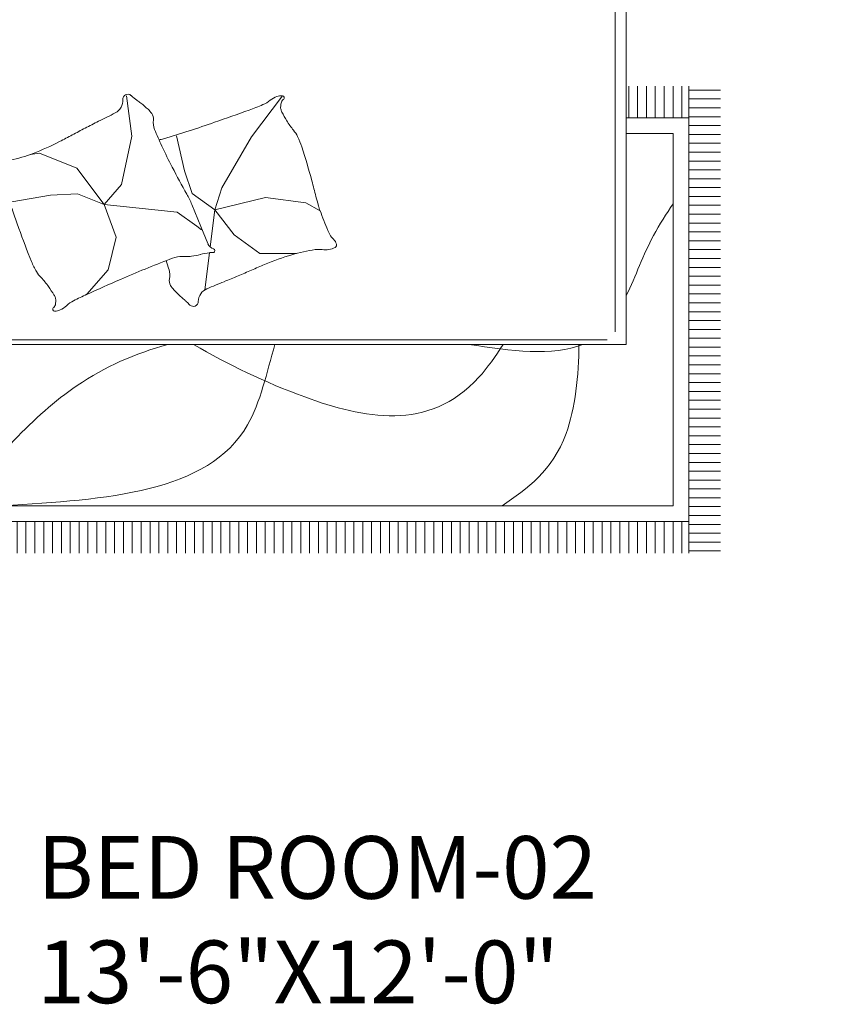
# Model space of a CAD drawing. Units: inches. Extents: x -7 to 1228, y -146 to 1091.
# Tile 30 of 88: x 680 to 744, y 367 to 446. Entities that reach past the tile are written whole.
import ezdxf

# ---------------------------------------------------------------- set-up
doc = ezdxf.new("R2010")
doc.units = ezdxf.units.IN
doc.layers.add('A-AREA-IDEN', color=7, linetype='Continuous', lineweight=18)
doc.layers.add('A-FURN', color=8, linetype='Continuous', lineweight=18)
doc.styles.add('DIM_FONT', font='SIMPLEX.shx', dxfattribs={"width": 0.8})
doc.styles.get("Standard").update_dxf_attribs({"font": 'arial.ttf'})

# ---------------------------------------------------------------- blocks, each defined once
blk = doc.blocks.new('A$C4F634EDD')
for p, q in [((0, 2.6295), (0, 2.2295)), ((0.5, 2.6295), (0, 2.6295)), ((0.5, 2.6295), (2.3, 2.6295)), ((0.5, 0.5295), (0.5, 2.6295)), ((0.5, 2.2295), (0.5, 2.6295)), ((2.3, 2.6295), (2.3, 0.5295)), ((2.3, 2.6295), (2.8, 2.6295)), ((2.3, 2.2295), (2.3, 2.6295)), ((2.8, 2.6295), (2.8, 2.2295)), ((0.5, 2.5771), (2.3, 2.5771)), ((2.392, 2.5115), (2.5692, 2.5765)), ((2.5692, 2.5765), (2.574, 2.5743)), ((0.2457, 2.5697), (0.2457, 2.4733)), ((2.4985, 2.5445), (2.5516, 2.564)), ((2.5062, 2.5454), (2.5487, 2.561)), ((2.5483, 2.5347), (2.5487, 2.561)), ((2.5487, 2.561), (2.5571, 2.56)), ((2.5615, 2.5536), (2.5514, 2.5318)), ((2.5516, 2.564), (2.5637, 2.5584)), ((2.5571, 2.56), (2.5615, 2.5536)), ((2.5615, 2.5536), (2.5791, 2.5058)), ((2.5637, 2.5584), (2.6418, 2.3458)), ((2.574, 2.5743), (2.6638, 2.3298)), ((2.4946, 2.5331), (2.4985, 2.5445)), ((2.5734, 2.3187), (2.4946, 2.5331)), ((2.5062, 2.5454), (2.5004, 2.5392)), ((2.5004, 2.5392), (2.5013, 2.5315)), ((2.5013, 2.5315), (2.5188, 2.4836)), ((2.5013, 2.5315), (2.5231, 2.5214)), ((2.5235, 2.5256), (2.5062, 2.5454)), ((2.5231, 2.5214), (2.5235, 2.5256)), ((2.5483, 2.5347), (2.5235, 2.5256)), ((2.5514, 2.5318), (2.5483, 2.5347)), ((2.5807, 2.4521), (2.5514, 2.5318)), ((2.3898, 2.5066), (2.392, 2.5115)), ((2.4795, 2.2621), (2.3898, 2.5066)), ((2.412, 2.5007), (2.4634, 2.5196)), ((2.4361, 2.4352), (2.412, 2.5007)), ((2.4634, 2.5196), (2.4875, 2.454)), ((2.4842, 2.5232), (2.47, 2.518)), ((2.47, 2.518), (2.472, 2.5127)), ((2.472, 2.5127), (2.4862, 2.5179)), ((2.4881, 2.5126), (2.4739, 2.5074)), ((2.4739, 2.5074), (2.4759, 2.502)), ((2.4759, 2.502), (2.4901, 2.5073)), ((2.492, 2.5019), (2.4778, 2.4967)), ((2.4862, 2.5179), (2.4842, 2.5232)), ((2.4901, 2.5073), (2.4881, 2.5126)), ((2.494, 2.4966), (2.492, 2.5019)), ((2.5523, 2.4417), (2.5231, 2.5214)), ((2.5791, 2.5058), (2.5788, 2.4956)), ((2.4778, 2.4967), (2.4798, 2.4914)), ((2.4798, 2.4914), (2.494, 2.4966)), ((2.4959, 2.4913), (2.4817, 2.4861)), ((2.4817, 2.4861), (2.4837, 2.4808)), ((2.4837, 2.4808), (2.4979, 2.486)), ((2.4998, 2.4807), (2.4856, 2.4755)), ((2.4856, 2.4755), (2.4876, 2.4702)), ((2.4876, 2.4702), (2.5018, 2.4754)), ((2.4979, 2.486), (2.4959, 2.4913)), ((2.5018, 2.4754), (2.4998, 2.4807)), ((2.5188, 2.4836), (2.5256, 2.4761)), ((2.5256, 2.4761), (2.5342, 2.4692)), ((2.5788, 2.4956), (2.5767, 2.4848)), ((2.5767, 2.4848), (2.5795, 2.4717)), ((2.4875, 2.454), (2.4361, 2.4352)), ((2.5037, 2.47), (2.4895, 2.4648)), ((2.4895, 2.4648), (2.4915, 2.4595)), ((2.4915, 2.4595), (2.5057, 2.4647)), ((2.5057, 2.4647), (2.5037, 2.47)), ((2.5342, 2.4692), (2.5405, 2.4574)), ((2.5405, 2.4574), (2.547, 2.4397)), ((2.5795, 2.4717), (2.586, 2.454)), ((2.5807, 2.4521), (2.6158, 2.3564)), ((2.5984, 2.4204), (2.586, 2.454)), ((2.4634, 2.4211), (2.474, 2.425)), ((2.474, 2.425), (2.4779, 2.4143)), ((2.4811, 2.4276), (2.4917, 2.4315)), ((2.485, 2.4169), (2.4811, 2.4276)), ((2.4917, 2.4315), (2.4956, 2.4208)), ((2.5594, 2.4061), (2.547, 2.4397)), ((2.5523, 2.4417), (2.5875, 2.346)), ((0.0957, 2.4197), (0.192, 2.4197)), ((0.2994, 2.4197), (0.3957, 2.4197)), ((2.4457, 2.4146), (2.4563, 2.4185)), ((2.4496, 2.4039), (2.4457, 2.4146)), ((2.4602, 2.4078), (2.4496, 2.4039)), ((2.4563, 2.4185), (2.4602, 2.4078)), ((2.4673, 2.4104), (2.4634, 2.4211)), ((2.4779, 2.4143), (2.4673, 2.4104)), ((2.4706, 2.4016), (2.4812, 2.4055)), ((2.4745, 2.3909), (2.4706, 2.4016)), ((2.4812, 2.4055), (2.4851, 2.3949)), ((2.4956, 2.4208), (2.485, 2.4169)), ((2.4883, 2.4081), (2.4989, 2.412)), ((2.4922, 2.3975), (2.4883, 2.4081)), ((2.5028, 2.4014), (2.4922, 2.3975)), ((2.4989, 2.412), (2.5028, 2.4014)), ((2.5622, 2.393), (2.5594, 2.4061)), ((2.6047, 2.4086), (2.5984, 2.4204)), ((2.6133, 2.4017), (2.6047, 2.4086)), ((2.6201, 2.3941), (2.6133, 2.4017)), ((2.4528, 2.3951), (2.4635, 2.399)), ((2.4567, 2.3844), (2.4528, 2.3951)), ((2.4674, 2.3883), (2.4567, 2.3844)), ((2.46, 2.3756), (2.4706, 2.3795)), ((2.4639, 2.365), (2.46, 2.3756)), ((2.4635, 2.399), (2.4674, 2.3883)), ((2.4706, 2.3795), (2.4745, 2.3689)), ((2.4851, 2.3949), (2.4745, 2.3909)), ((2.4777, 2.3821), (2.4883, 2.386)), ((2.4816, 2.3715), (2.4777, 2.3821)), ((2.4922, 2.3754), (2.4816, 2.3715)), ((2.4883, 2.386), (2.4922, 2.3754)), ((2.4954, 2.3886), (2.5061, 2.3925)), ((2.4993, 2.378), (2.4954, 2.3886)), ((2.51, 2.3819), (2.4993, 2.378)), ((2.5061, 2.3925), (2.51, 2.3819)), ((2.5238, 2.3769), (2.538, 2.3821)), ((2.5277, 2.3663), (2.5238, 2.3769)), ((2.538, 2.3821), (2.5419, 2.3715)), ((2.5598, 2.372), (2.5601, 2.3822)), ((2.5601, 2.3822), (2.5622, 2.393)), ((2.6376, 2.3463), (2.6201, 2.3941)), ((2.6499, 2.3979), (2.6397, 2.3953)), ((2.6417, 2.39), (2.6488, 2.391)), ((2.6488, 2.391), (2.6538, 2.3895)), ((2.6551, 2.397), (2.6499, 2.3979)), ((2.6538, 2.3895), (2.6596, 2.388)), ((2.6627, 2.392), (2.6551, 2.397)), ((2.6596, 2.388), (2.6626, 2.3867)), ((2.6626, 2.3867), (2.6662, 2.388)), ((2.6692, 2.394), (2.6627, 2.392)), ((2.6662, 2.388), (2.6632, 2.3828)), ((2.6632, 2.3828), (2.6736, 2.3744)), ((2.6736, 2.3944), (2.6692, 2.394)), ((2.6765, 2.391), (2.6736, 2.3944)), ((2.6742, 2.3795), (2.6765, 2.391)), ((2.6824, 2.3858), (2.6742, 2.3795)), ((2.6873, 2.3815), (2.6824, 2.3858)), ((2.6853, 2.369), (2.6873, 2.3815)), ((2.6946, 2.376), (2.6853, 2.369)), ((2.6995, 2.3713), (2.6946, 2.376)), ((0.2457, 2.366), (0.2457, 2.2697)), ((2.4745, 2.3689), (2.4639, 2.365)), ((2.4672, 2.3561), (2.4778, 2.36)), ((2.4711, 2.3455), (2.4672, 2.3561)), ((2.4778, 2.36), (2.4817, 2.3494)), ((2.4849, 2.3626), (2.4955, 2.3665)), ((2.4888, 2.352), (2.4849, 2.3626)), ((2.4994, 2.3559), (2.4888, 2.352)), ((2.4955, 2.3665), (2.4994, 2.3559)), ((2.5026, 2.3691), (2.5132, 2.373)), ((2.5065, 2.3585), (2.5026, 2.3691)), ((2.5171, 2.3624), (2.5065, 2.3585)), ((2.5132, 2.373), (2.5171, 2.3624)), ((2.5419, 2.3715), (2.5277, 2.3663)), ((2.5774, 2.3242), (2.5598, 2.372)), ((2.6154, 2.3522), (2.5905, 2.3431)), ((2.6158, 2.3564), (2.6154, 2.3522)), ((2.6154, 2.3522), (2.6327, 2.3324)), ((2.6376, 2.3463), (2.6158, 2.3564)), ((2.6736, 2.3744), (2.6922, 2.3593)), ((2.6922, 2.3593), (2.7051, 2.3473)), ((2.695, 2.3603), (2.6995, 2.3713)), ((2.7031, 2.3682), (2.695, 2.3603)), ((2.7096, 2.3616), (2.7031, 2.3682)), ((2.7062, 2.351), (2.7096, 2.3616)), ((2.7147, 2.3578), (2.7062, 2.351)), ((2.7214, 2.3517), (2.7147, 2.3578)), ((2.7196, 2.34), (2.7214, 2.3517)), ((0, 2.3301), (0.5, 2.3301)), ((2.8, 2.3301), (2.3, 2.3301)), ((2.4817, 2.3494), (2.4711, 2.3455)), ((2.5774, 2.3242), (2.5875, 2.346)), ((2.5875, 2.346), (2.5905, 2.3431)), ((2.5905, 2.3431), (2.5901, 2.3168)), ((2.613, 2.3312), (2.6077, 2.3293)), ((2.6077, 2.3293), (2.6135, 2.3141)), ((2.6192, 2.3174), (2.613, 2.3312)), ((2.6153, 2.3261), (2.6327, 2.3324)), ((2.6369, 2.332), (2.6161, 2.3243)), ((2.6616, 2.3249), (2.6234, 2.3109)), ((2.6327, 2.3324), (2.6385, 2.3386)), ((2.6418, 2.3458), (2.6369, 2.332)), ((2.6385, 2.3386), (2.6376, 2.3463)), ((2.6638, 2.3298), (2.6616, 2.3249)), ((2.7051, 2.3473), (2.7079, 2.3475)), ((2.7079, 2.3475), (2.7079, 2.3443)), ((2.7079, 2.3443), (2.727, 2.3277)), ((2.7286, 2.3466), (2.7196, 2.34)), ((2.727, 2.3277), (2.7512, 2.2983)), ((2.7346, 2.3423), (2.7286, 2.3466)), ((2.732, 2.3295), (2.7346, 2.3423)), ((2.7423, 2.3345), (2.732, 2.3295)), ((2.7406, 2.3172), (2.7495, 2.325)), ((2.7495, 2.325), (2.7423, 2.3345)), ((2.6172, 2.3086), (2.4844, 2.2599)), ((2.5362, 2.305), (2.5185, 2.2985)), ((2.5401, 2.2944), (2.5362, 2.305)), ((2.561, 2.3141), (2.5433, 2.3076)), ((2.5433, 2.3076), (2.5472, 2.297)), ((2.5472, 2.297), (2.5649, 2.3035)), ((2.5649, 2.3035), (2.561, 2.3141)), ((2.5855, 2.3131), (2.5734, 2.3187)), ((2.5818, 2.3178), (2.5774, 2.3242)), ((2.5901, 2.3168), (2.5818, 2.3178)), ((2.6104, 2.3222), (2.5855, 2.3131)), ((2.5901, 2.3168), (2.6097, 2.324)), ((2.6135, 2.3141), (2.6244, 2.2977)), ((2.626, 2.3069), (2.6192, 2.3174)), ((2.6365, 2.2916), (2.626, 2.3069)), ((2.7519, 2.3218), (2.7406, 2.3172)), ((2.7575, 2.3144), (2.7519, 2.3218)), ((2.7526, 2.3045), (2.7575, 2.3144)), ((2.7622, 2.308), (2.7526, 2.3045)), ((2.7673, 2.2997), (2.7622, 2.308)), ((2.5114, 2.2959), (2.4936, 2.2894)), ((2.4936, 2.2894), (2.4976, 2.2788)), ((2.4976, 2.2788), (2.5153, 2.2853)), ((2.5153, 2.2853), (2.5114, 2.2959)), ((2.5185, 2.2985), (2.5224, 2.2879)), ((2.5224, 2.2879), (2.5401, 2.2944)), ((2.6244, 2.2977), (2.6349, 2.2825)), ((2.6349, 2.2825), (2.638, 2.273)), ((2.6407, 2.2834), (2.6365, 2.2916)), ((2.6438, 2.2739), (2.6407, 2.2834)), ((2.7512, 2.2983), (2.756, 2.2695)), ((2.7574, 2.2924), (2.7673, 2.2997)), ((2.7687, 2.2905), (2.7574, 2.2924)), ((2.7587, 2.279), (2.7699, 2.2828)), ((2.7708, 2.2725), (2.7587, 2.279)), ((2.7699, 2.2828), (2.7687, 2.2905)), ((0.5953, 2.1912), (0.616, 2.2738)), ((1.4546, 2.1912), (1.4752, 2.2738)), ((2.4844, 2.2599), (2.4795, 2.2621)), ((2.6399, 2.2712), (2.6374, 2.2659)), ((2.6374, 2.2659), (2.6398, 2.257)), ((2.638, 2.273), (2.6399, 2.2712)), ((2.6398, 2.257), (2.6509, 2.259)), ((2.6509, 2.259), (2.6431, 2.2492)), ((2.6519, 2.2716), (2.6438, 2.2739)), ((2.6535, 2.2628), (2.6519, 2.2716)), ((2.6636, 2.2409), (2.6535, 2.2628)), ((2.756, 2.2695), (2.7459, 2.2483)), ((2.7529, 2.2505), (2.7645, 2.2498)), ((2.7607, 2.2424), (2.7529, 2.2505)), ((2.759, 2.2637), (2.7706, 2.2643)), ((2.7676, 2.2559), (2.759, 2.2637)), ((2.7645, 2.2498), (2.7676, 2.2559)), ((2.7706, 2.2643), (2.7708, 2.2725)), ((0, 2.2295), (0.5, 2.2295)), ((2.8, 2.2295), (2.3, 2.2295)), ((2.6431, 2.2492), (2.6473, 2.2398)), ((2.6473, 2.2398), (2.6592, 2.2429)), ((2.6592, 2.2429), (2.6521, 2.2314)), ((2.6521, 2.2314), (2.6598, 2.2248)), ((2.6598, 2.2248), (2.6697, 2.2309)), ((2.6836, 2.2287), (2.6636, 2.2409)), ((2.6697, 2.2309), (2.6684, 2.219)), ((2.7063, 2.2256), (2.6836, 2.2287)), ((2.7284, 2.2317), (2.7063, 2.2256)), ((2.7255, 2.2152), (2.7242, 2.2265)), ((2.7242, 2.2265), (2.7324, 2.2165)), ((2.7459, 2.2483), (2.7284, 2.2317)), ((2.7386, 2.2208), (2.7354, 2.2306)), ((2.7354, 2.2306), (2.7462, 2.2264)), ((2.7509, 2.2314), (2.7459, 2.2418)), ((2.7459, 2.2418), (2.7568, 2.2352)), ((2.7462, 2.2264), (2.7509, 2.2314)), ((2.7568, 2.2352), (2.7607, 2.2424)), ((2.6684, 2.219), (2.6761, 2.2145)), ((2.6761, 2.2145), (2.6821, 2.2237)), ((2.6821, 2.2237), (2.6843, 2.2135)), ((2.6843, 2.2135), (2.6927, 2.2117)), ((2.6927, 2.2117), (2.6986, 2.222)), ((2.6986, 2.222), (2.7019, 2.2098)), ((2.7019, 2.2098), (2.7102, 2.2104)), ((2.7102, 2.2104), (2.7113, 2.2218)), ((2.7113, 2.2218), (2.7192, 2.2137)), ((2.7192, 2.2137), (2.7255, 2.2152)), ((2.7324, 2.2165), (2.7386, 2.2208)), ((0.5878, 2.1612), (0.5953, 2.1912)), ((1.4471, 2.1612), (1.4546, 2.1912)), ((1.5035, 2.141), (0.5458, 2.141)), ((1.5035, 2.141), (2.2716, 1.7136)), ((0.5258, 2.121), (0.5258, 0.5617)), ((1.576, 1.9433), (1.5624, 1.8479)), ((0.5458, 1.8684), (1.5653, 1.8684)), ((1.5624, 1.8479), (1.5641, 1.7178)), ((2.2716, 0.5617), (2.2716, 1.7136)), ((0.2586, 1.1753), (0.3386, 1.1753)), ((0.3386, 0), (0.3386, 1.1852)), ((0.3486, 1.1052), (0.3486, 1.1852)), ((0.3711, 1.1052), (0.3711, 1.1852)), ((0.3936, 1.1052), (0.3936, 1.1852)), ((0.4161, 1.1052), (0.4161, 1.1852)), ((0.4386, 1.1052), (0.4386, 1.1852)), ((0.4611, 1.1052), (0.4611, 1.1852)), ((0.4836, 1.1052), (0.4836, 1.1852)), ((2.3061, 1.1052), (2.3061, 1.1852)), ((2.3286, 1.1052), (2.3286, 1.1852)), ((2.3511, 1.1052), (2.3511, 1.1852)), ((2.3736, 1.1052), (2.3736, 1.1852)), ((2.3961, 1.1052), (2.3961, 1.1852)), ((2.4186, 1.1052), (2.4186, 1.1852)), ((2.4411, 1.1052), (2.4411, 1.1852)), ((2.4588, 1.1852), (2.4588, 0)), ((2.4588, 1.1753), (2.5388, 1.1753)), ((0.2586, 1.1528), (0.3386, 1.1528)), ((1.031, 1.1612), (1.0448, 1.0581)), ((1.4276, 1.1611), (1.3484, 1.0571)), ((2.4588, 1.1528), (2.5388, 1.1528)), ((0.2586, 1.1303), (0.3386, 1.1303)), ((2.4588, 1.1303), (2.5388, 1.1303)), ((0.2586, 1.1078), (0.3386, 1.1078)), ((0.3386, 1.1052), (0.5, 1.1052)), ((2.3, 1.1052), (2.4588, 1.1052)), ((2.4588, 1.1078), (2.5388, 1.1078)), ((0.2586, 1.0853), (0.3386, 1.0853)), ((2.4588, 1.0853), (2.5388, 1.0853)), ((0.2586, 1.0628), (0.3386, 1.0628)), ((0.3786, 1.0652), (0.5, 1.0652)), ((0.3786, 0.12), (0.3786, 1.0652)), ((1.0448, 1.0581), (1.019, 0.936)), ((1.1784, 0.9702), (1.1586, 1.0591)), ((1.3484, 1.0571), (1.2733, 0.9268)), ((2.3, 1.0652), (2.4188, 1.0652)), ((2.4188, 1.0652), (2.4188, 0.12)), ((2.4588, 1.0628), (2.5388, 1.0628)), ((0.2586, 1.0403), (0.3386, 1.0403)), ((2.4588, 1.0403), (2.5388, 1.0403)), ((0.2586, 1.0178), (0.3386, 1.0178)), ((0.8108, 1.0151), (0.7868, 1.0117)), ((0.9054, 0.9773), (0.8108, 1.0151)), ((2.4588, 1.0178), (2.5388, 1.0178)), ((0.2586, 0.9953), (0.3386, 0.9953)), ((0.9743, 0.8845), (0.9054, 0.9773)), ((2.4588, 0.9953), (2.5388, 0.9953)), ((0.2586, 0.9728), (0.3386, 0.9728)), ((0.2586, 0.9503), (0.3386, 0.9503)), ((1.1982, 0.9129), (1.1784, 0.9702)), ((2.4588, 0.9728), (2.5388, 0.9728)), ((2.4588, 0.9503), (2.5388, 0.9503)), ((0.2586, 0.9278), (0.3386, 0.9278)), ((1.019, 0.936), (0.9743, 0.8845)), ((1.2733, 0.9268), (1.2555, 0.8715)), ((2.4588, 0.9278), (2.5388, 0.9278)), ((0.2586, 0.9053), (0.3386, 0.9053)), ((0.8384, 0.9085), (0.7403, 0.8913)), ((0.9072, 0.912), (0.8384, 0.9085)), ((0.9743, 0.8845), (0.9072, 0.912)), ((1.2555, 0.8715), (1.1982, 0.9129)), ((1.2555, 0.8715), (1.384, 0.9031)), ((1.384, 0.9031), (1.4868, 0.8892)), ((2.4588, 0.9053), (2.5388, 0.9053)), ((0.2586, 0.8828), (0.3386, 0.8828)), ((0.7403, 0.8913), (0.737, 0.8849)), ((0.9743, 0.8845), (1.0052, 0.802)), ((0.9743, 0.8845), (1.16, 0.8656)), ((1.1973, 0.8853), (1.2203, 0.829)), ((1.4868, 0.8892), (1.5228, 0.8692)), ((2.4588, 0.8828), (2.5388, 0.8828)), ((0.2586, 0.8603), (0.3386, 0.8603)), ((1.16, 0.8656), (1.2099, 0.8295)), ((1.2555, 0.8715), (1.2437, 0.7773)), ((1.2555, 0.8715), (1.3049, 0.8082)), ((2.4588, 0.8603), (2.5388, 0.8603)), ((0.2586, 0.8378), (0.3386, 0.8378)), ((1.2099, 0.8295), (1.222, 0.8209)), ((1.2203, 0.829), (1.2381, 0.7855)), ((2.4588, 0.8378), (2.5388, 0.8378)), ((0.2586, 0.8153), (0.3386, 0.8153)), ((1.0052, 0.802), (0.9846, 0.7194)), ((1.3049, 0.8082), (1.3701, 0.7608)), ((2.4588, 0.8153), (2.5388, 0.8153)), ((0.2586, 0.7928), (0.3386, 0.7928)), ((2.4588, 0.7928), (2.5388, 0.7928)), ((0.2586, 0.7703), (0.3386, 0.7703)), ((1.2419, 0.7626), (1.23, 0.668)), ((1.3701, 0.7608), (1.463, 0.7608)), ((2.4588, 0.7703), (2.5388, 0.7703)), ((0.2586, 0.7478), (0.3386, 0.7478)), ((0.2586, 0.7253), (0.3386, 0.7253)), ((2.4588, 0.7478), (2.5388, 0.7478)), ((2.4588, 0.7253), (2.5388, 0.7253)), ((0.2586, 0.7028), (0.3386, 0.7028)), ((0.9846, 0.7194), (0.931, 0.6569)), ((2.4588, 0.7028), (2.5388, 0.7028)), ((0.2586, 0.6803), (0.3386, 0.6803)), ((2.4588, 0.6803), (2.5388, 0.6803)), ((0.2586, 0.6578), (0.3386, 0.6578)), ((2.4588, 0.6578), (2.5388, 0.6578)), ((0.2586, 0.6353), (0.3386, 0.6353)), ((2.4588, 0.6353), (2.5388, 0.6353)), ((0.2586, 0.6128), (0.3386, 0.6128)), ((2.4588, 0.6128), (2.5388, 0.6128)), ((0.2586, 0.5903), (0.3386, 0.5903)), ((2.4588, 0.5903), (2.5388, 0.5903)), ((0.2586, 0.5678), (0.3386, 0.5678)), ((2.4588, 0.5678), (2.5388, 0.5678)), ((0.2586, 0.5453), (0.3386, 0.5453)), ((2.3, 0.5295), (0.5, 0.5295)), ((0.5458, 0.5417), (2.2516, 0.5417)), ((2.4588, 0.5453), (2.5388, 0.5453)), ((0.2586, 0.5228), (0.3386, 0.5228)), ((0.2586, 0.5003), (0.3386, 0.5003)), ((2.4588, 0.5228), (2.5388, 0.5228)), ((2.4588, 0.5003), (2.5388, 0.5003)), ((0.2586, 0.4778), (0.3386, 0.4778)), ((2.4588, 0.4778), (2.5388, 0.4778)), ((0.2586, 0.4553), (0.3386, 0.4553)), ((2.4588, 0.4553), (2.5388, 0.4553)), ((0.2586, 0.4328), (0.3386, 0.4328)), ((2.4588, 0.4328), (2.5388, 0.4328)), ((0.2586, 0.4103), (0.3386, 0.4103)), ((2.4588, 0.4103), (2.5388, 0.4103)), ((0.2586, 0.3878), (0.3386, 0.3878)), ((2.4588, 0.3878), (2.5388, 0.3878)), ((0.2586, 0.3653), (0.3386, 0.3653)), ((2.4588, 0.3653), (2.5388, 0.3653)), ((0.2586, 0.3428), (0.3386, 0.3428)), ((2.4588, 0.3428), (2.5388, 0.3428)), ((0.2586, 0.3203), (0.3386, 0.3203)), ((2.4588, 0.3203), (2.5388, 0.3203)), ((0.2586, 0.2978), (0.3386, 0.2978)), ((0.2586, 0.2753), (0.3386, 0.2753)), ((2.4588, 0.2978), (2.5388, 0.2978)), ((2.4588, 0.2753), (2.5388, 0.2753)), ((0.2586, 0.2528), (0.3386, 0.2528)), ((2.4588, 0.2528), (2.5388, 0.2528)), ((0.2586, 0.2303), (0.3386, 0.2303)), ((2.4588, 0.2303), (2.5388, 0.2303)), ((0.2586, 0.2078), (0.3386, 0.2078)), ((2.4588, 0.2078), (2.5388, 0.2078)), ((0.2586, 0.1853), (0.3386, 0.1853)), ((2.4588, 0.1853), (2.5388, 0.1853)), ((0.2586, 0.1628), (0.3386, 0.1628)), ((2.4588, 0.1628), (2.5388, 0.1628)), ((0.2586, 0.1403), (0.3386, 0.1403)), ((2.4588, 0.1403), (2.5388, 0.1403)), ((0.2586, 0.1178), (0.3386, 0.1178)), ((2.4188, 0.12), (0.3786, 0.12)), ((2.4588, 0.1178), (2.5388, 0.1178)), ((0.2586, 0.0953), (0.3386, 0.0953)), ((2.4588, 0.08), (0.3386, 0.08)), ((0.3486, 0), (0.3486, 0.08)), ((0.3711, 0), (0.3711, 0.08)), ((0.3936, 0), (0.3936, 0.08)), ((0.4161, 0), (0.4161, 0.08)), ((0.4386, 0), (0.4386, 0.08)), ((0.4611, 0), (0.4611, 0.08)), ((0.4836, 0), (0.4836, 0.08)), ((0.5061, 0), (0.5061, 0.08)), ((0.5286, 0), (0.5286, 0.08)), ((0.5511, 0), (0.5511, 0.08)), ((0.5736, 0), (0.5736, 0.08)), ((0.5961, 0), (0.5961, 0.08)), ((0.6186, 0), (0.6186, 0.08)), ((0.6411, 0), (0.6411, 0.08)), ((0.6636, 0), (0.6636, 0.08)), ((0.6861, 0), (0.6861, 0.08)), ((0.7086, 0), (0.7086, 0.08)), ((0.7311, 0), (0.7311, 0.08)), ((0.7536, 0), (0.7536, 0.08)), ((0.7761, 0), (0.7761, 0.08)), ((0.7986, 0), (0.7986, 0.08)), ((0.8211, 0), (0.8211, 0.08)), ((0.8436, 0), (0.8436, 0.08)), ((0.8661, 0), (0.8661, 0.08)), ((0.8886, 0), (0.8886, 0.08)), ((0.9111, 0), (0.9111, 0.08)), ((0.9336, 0), (0.9336, 0.08)), ((0.9561, 0), (0.9561, 0.08)), ((0.9786, 0), (0.9786, 0.08)), ((1.0011, 0), (1.0011, 0.08)), ((1.0236, 0), (1.0236, 0.08)), ((1.0461, 0), (1.0461, 0.08)), ((1.0686, 0), (1.0686, 0.08)), ((1.0911, 0), (1.0911, 0.08)), ((1.1136, 0), (1.1136, 0.08)), ((1.1361, 0), (1.1361, 0.08)), ((1.1586, 0), (1.1586, 0.08)), ((1.1811, 0), (1.1811, 0.08)), ((1.2036, 0), (1.2036, 0.08)), ((1.2261, 0), (1.2261, 0.08)), ((1.2486, 0), (1.2486, 0.08)), ((1.2711, 0), (1.2711, 0.08)), ((1.2936, 0), (1.2936, 0.08)), ((1.3161, 0), (1.3161, 0.08)), ((1.3386, 0), (1.3386, 0.08)), ((1.3611, 0), (1.3611, 0.08)), ((1.3836, 0), (1.3836, 0.08)), ((1.4061, 0), (1.4061, 0.08)), ((1.4286, 0), (1.4286, 0.08)), ((1.4511, 0), (1.4511, 0.08)), ((1.4736, 0), (1.4736, 0.08)), ((1.4961, 0), (1.4961, 0.08)), ((1.5186, 0), (1.5186, 0.08)), ((1.5411, 0), (1.5411, 0.08)), ((1.5636, 0), (1.5636, 0.08)), ((1.5861, 0), (1.5861, 0.08)), ((1.6086, 0), (1.6086, 0.08)), ((1.6311, 0), (1.6311, 0.08)), ((1.6536, 0), (1.6536, 0.08)), ((1.6761, 0), (1.6761, 0.08)), ((1.6986, 0), (1.6986, 0.08)), ((1.7211, 0), (1.7211, 0.08)), ((1.7436, 0), (1.7436, 0.08)), ((1.7661, 0), (1.7661, 0.08)), ((1.7886, 0), (1.7886, 0.08)), ((1.8111, 0), (1.8111, 0.08)), ((1.8336, 0), (1.8336, 0.08)), ((1.8561, 0), (1.8561, 0.08)), ((1.8786, 0), (1.8786, 0.08)), ((1.9011, 0), (1.9011, 0.08)), ((1.9236, 0), (1.9236, 0.08)), ((1.9461, 0), (1.9461, 0.08)), ((1.9686, 0), (1.9686, 0.08)), ((1.9911, 0), (1.9911, 0.08)), ((2.0136, 0), (2.0136, 0.08)), ((2.0361, 0), (2.0361, 0.08)), ((2.0586, 0), (2.0586, 0.08)), ((2.0811, 0), (2.0811, 0.08)), ((2.1036, 0), (2.1036, 0.08)), ((2.1261, 0), (2.1261, 0.08)), ((2.1486, 0), (2.1486, 0.08)), ((2.1711, 0), (2.1711, 0.08)), ((2.1936, 0), (2.1936, 0.08)), ((2.2161, 0), (2.2161, 0.08)), ((2.2386, 0), (2.2386, 0.08)), ((2.2611, 0), (2.2611, 0.08)), ((2.2836, 0), (2.2836, 0.08)), ((2.3061, 0), (2.3061, 0.08)), ((2.3286, 0), (2.3286, 0.08)), ((2.3511, 0), (2.3511, 0.08)), ((2.3736, 0), (2.3736, 0.08)), ((2.3961, 0), (2.3961, 0.08)), ((2.4186, 0), (2.4186, 0.08)), ((2.4411, 0), (2.4411, 0.08)), ((2.4588, 0.0953), (2.5388, 0.0953)), ((0.2586, 0.0728), (0.3386, 0.0728)), ((0.2586, 0.0503), (0.3386, 0.0503)), ((2.4588, 0.0728), (2.5388, 0.0728)), ((2.4588, 0.0503), (2.5388, 0.0503)), ((0.2586, 0.0278), (0.3386, 0.0278)), ((2.4588, 0.0278), (2.5388, 0.0278)), ((0.2586, 0.0053), (0.3386, 0.0053)), ((2.4588, 0.0053), (2.5388, 0.0053))]:
    blk.add_line(p, q)
for radius in [0.1222, 0.0865]:
    blk.add_circle((0.2457, 2.4197), radius)
for centre, radius, start, end in [((0.5848, 2.5274), 0.0131, 101.2724, 206.5805), ((0.5999, 2.4516), 0.0904, 90, 101.2724), ((0.5999, 2.3808), 0.1611, 81.5628, 90), ((0.5788, 2.2388), 0.3048, 74.256, 81.5628), ((0.7272, 2.7653), 0.2422, 254.256, 262.4531), ((0.7851, 3.2019), 0.6827, 262.4531, 270), ((0.7851, 3.5682), 1.049, 270, 276.0867), ((0.8402, 3.0514), 0.5293, 276.0867, 280.1899), ((1.1602, -8.1346), 10.6675, 90.30153, 91.21582), ((1.1169, 2.2433), 0.2897, 85.1982, 92.5386), ((1.2142, 3.4021), 0.8732, 265.1982, 269.4243), ((1.3082, 2.3102), 0.234, 110.8603, 117.2396), ((1.2204, 4.0232), 1.4943, 269.4243, 271.9079), ((1.2995, 2.4357), 0.0992, 105.9352, 126.0864), ((1.2429, 3.3501), 0.8208, 271.9079, 275.2592), ((1.2995, 2.4357), 0.0992, 85.7841, 105.9352), ((1.3132, 2.5864), 0.0539, 275.2592, 300.6513), ((1.3554, 2.5152), 0.0289, 85.6975, 120.6513), ((1.3556, 2.519), 0.0251, 68.2117, 85.6975), ((1.3739, 2.5288), 0.0156, 158.0096, 201.421), ((1.3634, 2.533), 0.00428, 78.1069, 158.0096), ((1.3647, 2.5395), 0.00232, 258.1069, 19.564), ((1.3637, 2.5391), 0.00342, 19.564, 68.2117), ((1.444, 2.5274), 0.0131, 101.2724, 206.5805), ((1.4591, 2.4516), 0.0904, 90, 101.2724), ((1.4591, 2.3808), 0.1611, 81.5628, 90), ((1.438, 2.2388), 0.3048, 74.256, 81.5628), ((1.5865, 2.7653), 0.2422, 254.256, 262.4531), ((1.6443, 3.2019), 0.6827, 262.4531, 270), ((1.6443, 3.5682), 1.049, 270, 276.0867), ((1.4785, 15.4878), 12.9656, 271.22425, 272.05324), ((1.97, 2.3805), 0.1524, 92.5386, 100.1899), ((1.9761, 2.2433), 0.2897, 85.1982, 92.5386), ((2.0734, 3.4021), 0.8732, 265.1982, 269.4243), ((2.1674, 2.3102), 0.234, 110.8603, 117.2396), ((2.0797, 4.0232), 1.4943, 269.4243, 271.9079), ((2.1588, 2.4357), 0.0992, 105.9352, 126.0864), ((2.1021, 3.3501), 0.8208, 271.9079, 275.2592), ((2.1588, 2.4357), 0.0992, 85.7841, 105.9352), ((2.1724, 2.5864), 0.0539, 275.2592, 300.6513), ((2.2146, 2.5152), 0.0289, 85.6975, 120.6513), ((2.2149, 2.519), 0.0251, 68.2117, 85.6975), ((2.2331, 2.5288), 0.0156, 158.0096, 201.421), ((2.2226, 2.533), 0.00428, 78.1069, 158.0096), ((2.224, 2.5395), 0.00232, 258.1069, 19.564), ((2.2229, 2.5391), 0.00342, 19.564, 68.2117), ((0.6036, 2.5368), 0.0342, 206.5805, 265.5998), ((1.0898, 2.4496), 0.4918, 173.7676, 180), ((0.5368, 2.3783), 0.1399, 45.0976, 62.7964), ((1.4317, 2.2032), 0.3916, 128.3886, 133.8115), ((1.2362, 2.45), 0.0768, 117.2396, 128.3886), ((1.2995, 2.4357), 0.0992, 126.0864, 143.8234), ((1.1177, 2.5413), 0.246, 347.8905, 351.8665), ((1.3288, 2.5111), 0.0328, 351.8665, 21.421), ((1.4628, 2.5368), 0.0342, 206.5805, 265.5998), ((1.949, 2.4496), 0.4918, 173.7676, 180), ((2.291, 2.2032), 0.3916, 128.3886, 133.8115), ((2.0954, 2.45), 0.0768, 117.2396, 128.3886), ((2.1588, 2.4357), 0.0992, 126.0864, 143.8234), ((1.977, 2.5413), 0.246, 347.8905, 351.8665), ((2.1881, 2.5111), 0.0328, 351.8665, 21.421), ((0.5462, 2.4142), 0.0899, 41.4429, 53.7359), ((0.5368, 2.3783), 0.1399, 27.3988, 45.0976), ((1.3165, 2.3233), 0.2252, 133.8115, 140.9651), ((1.2995, 2.4357), 0.0992, 143.8234, 161.5603), ((1.5522, 2.448), 0.1983, 167.8905, 172.3191), ((2.1757, 2.3233), 0.2252, 133.8115, 140.9651), ((2.1588, 2.4357), 0.0992, 143.8234, 161.5603), ((2.4114, 2.448), 0.1983, 167.8905, 172.3191), ((0.5741, 2.4389), 0.0526, 25.3551, 41.4429), ((0.4851, 2.3967), 0.1511, 21.8149, 25.3551), ((0.4345, 2.3765), 0.2056, 18.7799, 21.8149), ((1.3127, 2.3625), 0.2002, 151.6832, 156.9972), ((1.1799, 2.4341), 0.0493, 140.9651, 151.6832), ((2.2605, 2.3525), 0.9131, 172.3191, 176.6313), ((2.1719, 2.3625), 0.2002, 151.6832, 156.9972), ((2.0391, 2.4341), 0.0493, 140.9651, 151.6832), ((3.1198, 2.3525), 0.9131, 172.3191, 176.6313), ((0.8019, 2.4496), 0.204, 180, 189.6844), ((0.576, 2.4246), 0.0562, 0, 18.7799), ((0.5368, 2.3783), 0.1399, 16.515, 27.3988), ((1.6611, 2.4496), 0.204, 180, 189.6844), ((1.4703, 2.5637), 0.882, 189.6844, 192.1984), ((0.5406, 2.4246), 0.0915, 345.3149, 0), ((0.5368, 2.3783), 0.1399, 5.6311, 16.515), ((2.0266, 2.3663), 0.6787, 176.6313, 181.6331), ((2.3295, 2.5637), 0.882, 189.6844, 192.1984), ((2.8858, 2.3663), 0.6787, 176.6313, 181.6331), ((0.2982, 2.3103), 0.3171, 8.0051, 12.1984), ((1.1575, 2.3103), 0.3171, 8.0051, 12.1984), ((-0.0401, 2.2627), 0.6588, 2.6649, 8.0051), ((0.8191, 2.2627), 0.6588, 2.6649, 8.0051), ((2.7128, 2.3859), 1.3652, 181.6331, 183.055), ((3.5721, 2.3859), 1.3652, 181.6331, 183.055), ((14.9657, 3.0398), 13.6356, 183.05496, 183.50486), ((15.8249, 3.0398), 13.6356, 183.05496, 183.50486), ((0.5503, 2.2902), 0.0677, 345.9548, 2.6649), ((1.4096, 2.2902), 0.0677, 345.9548, 2.6649), ((1.1303, 1.9835), 0.2721, 85.9172, 93.5552), ((1.1455, 2.197), 0.058, 69.3257, 85.9172), ((0.9871, 1.7772), 0.5066, 65.6735, 69.3257), ((0.6058, 0.9338), 1.4323, 63.5015, 65.6735), ((0.473, 2.8815), 0.7387, 291.6577, 293.4844), ((0.473, 2.8815), 0.7387, 293.4844, 295.3111), ((1.1054, 1.9358), 0.3126, 57.865, 63.5015), ((0.8841, 1.5835), 0.7286, 54.1737, 57.865), ((1.6762, 2.2258), 0.3212, 183.5049, 189.9984), ((1.3322, 2.8815), 0.7387, 291.6577, 293.4844), ((1.3322, 2.8815), 0.7387, 293.4844, 295.3111), ((2.5355, 2.2258), 0.3212, 183.5049, 189.9984), ((0.6807, 2.0561), 0.1197, 96.4341, 107.3864), ((0.6836, 2.0301), 0.1459, 78.4414, 96.4341), ((0.473, 2.8815), 0.7387, 287.1982, 289.428), ((0.473, 2.8815), 0.7387, 289.428, 291.6577), ((1.2501, -19.8405), 22.0183, 90.37908, 91.01965), ((1.2012, -3.5404), 5.7185, 89.7135, 90.9704), ((1.224, 1.0141), 1.164, 86.426, 89.7135), ((1.2875, 2.0302), 0.1459, 77.131, 86.426), ((1.5399, 2.0561), 0.1197, 96.4341, 107.3864), ((1.5429, 2.0301), 0.1459, 78.4414, 96.4341), ((1.3322, 2.8815), 0.7387, 287.1982, 289.428), ((1.3322, 2.8815), 0.7387, 289.428, 291.6577), ((2.1093, -19.8405), 22.0183, 90.37908, 91.01965), ((2.0605, -3.5404), 5.7185, 89.7135, 90.9704), ((2.0833, 1.0141), 1.164, 86.426, 89.7135), ((2.1467, 2.0302), 0.1459, 77.131, 86.426), ((0.5887, 2.1609), 0.000917, 165.9551, 274.0829), ((0.5695, 2.4301), 0.2708, 274.0829, 279.4841), ((0.5763, 2.3896), 0.2297, 279.4841, 287.3864), ((0.759, 2.3985), 0.2301, 258.4414, 272.7491), ((0.7026, 3.5718), 1.4048, 272.7491, 274.6176), ((0.9136, 0.9591), 1.2165, 92.6096, 94.6176), ((1.3099, 2.1283), 0.0453, 62.7159, 77.131), ((1.3658, 2.2367), 0.0767, 242.7159, 253.7788), ((1.3688, 2.247), 0.0875, 253.7788, 262.8796), ((1.3581, 2.1615), 0.00132, 262.8796, 343.3022), ((1.3409, 2.1667), 0.0193, 343.3022, 9.9984), ((1.448, 2.1609), 0.000917, 165.9551, 274.0829), ((1.4288, 2.4301), 0.2708, 274.0829, 279.4841), ((1.4355, 2.3896), 0.2297, 279.4841, 287.3864), ((1.6182, 2.3985), 0.2301, 258.4414, 272.7491), ((1.5619, 3.5718), 1.4048, 272.7491, 274.6176), ((1.7729, 0.9591), 1.2165, 92.6096, 94.6176), ((2.1691, 2.1283), 0.0453, 62.7159, 77.131), ((2.2251, 2.2367), 0.0767, 242.7159, 253.7788), ((2.2281, 2.247), 0.0875, 253.7788, 262.8796), ((2.2174, 2.1615), 0.00132, 262.8796, 343.3022), ((2.2001, 2.1667), 0.0193, 343.3022, 9.9984), ((0.5458, 2.121), 0.02, 90, 180), ((1.2147, 1.9017), 0.3751, 20.1488, 39.6445), ((1.3977, 1.9688), 0.1801, 351.8644, 20.1488), ((0.5458, 1.8884), 0.02, 180, 270), ((0.6102, 18.0525), 16.3521, 273.75703, 274.62393), ((1.4194, 4.2174), 2.5158, 281.6741, 283.1904), ((2.0378, 1.5789), 0.1942, 97.7304, 103.1904), ((2.0195, 1.7137), 0.0581, 79.2724, 97.7304), ((1.2737, -2.2227), 4.0646, 77.0745, 79.2724), ((1.0582, 5.4638), 3.7801, 277.692, 279.495), ((2.0359, 1.0981), 0.6574, 74.0648, 77.0745), ((1.7125, -0.0344), 1.8351, 72.2636, 74.0648), ((0.9863, 1.1494), 0.0359, 297.2902, 3.2455), ((1.0348, 1.1521), 0.0127, 51.1864, 183.2455), ((0.9991, 1.1077), 0.0697, 45.8726, 51.1864), ((1.0791, 1.1902), 0.0452, 225.8726, 232.4713), ((1.2846, 1.4577), 0.3825, 232.4713, 233.7837), ((1.4338, 1.1026), 0.0601, 110.3452, 128.5854), ((1.4251, 1.1259), 0.0352, 86.0516, 110.3452), ((1.4376, 1.1398), 0.0142, 126.5792, 169.5926), ((1.4273, 1.1567), 0.00443, 13.2808, 86.0516), ((1.4254, 1.1562), 0.0063, 306.5792, 13.2808), ((0.6683, 0.6162), 0.6605, 52.7849, 53.7837), ((0.9362, 0.9689), 0.2176, 46.4776, 52.7849), ((1.0327, 1.0706), 0.0774, 35.8936, 46.4776), ((1.0543, 1.9106), 0.8371, 290.1287, 292.7069), ((1.3469, 1.2115), 0.0792, 292.7069, 308.5854), ((1.4996, 1.1284), 0.0771, 169.5926, 177.2714), ((1.4378, 1.1314), 0.0153, 177.2714, 194.5709), ((1.4611, 1.1374), 0.0393, 194.5709, 206.8179), ((-0.4173, 3.8699), 3.0972, 296.4147, 297.2902), ((1.0771, 1.1027), 0.0226, 351.9508, 35.8936), ((-0.4107, 5.9078), 5.0942, 289.0836, 290.1287), ((1.7401, 1.2785), 0.352, 206.8179, 210.9056), ((3.744, -4.3336), 6.1019, 117.49986, 117.84822), ((1.8575, -0.7096), 2.0162, 116.4147, 117.4999), ((1.1449, 1.0931), 0.0458, 171.9508, 202.4162), ((2.032, 1.4591), 1.0054, 202.4162, 205.0529), ((0.2266, 4.0657), 3.145, 286.6085, 289.0836), ((1.6045, 1.1973), 0.194, 210.9056, 219.7005), ((-1.8336, 6.2238), 5.8383, 297.49208, 297.84822), ((1.0922, 1.1636), 0.1166, 280.7366, 286.6085), ((1.3929, 1.0217), 0.081, 26.0735, 39.7005), ((1.2892, 0.9709), 0.1965, 17.8396, 26.0735), ((0.5736, 1.5979), 0.6236, 290.7486, 297.4921), ((2.6493, 1.7476), 1.6868, 205.0529, 207.0884), ((-0.4304, 0.4175), 2.003, 15.2625, 17.8396), ((0.6422, 1.4168), 0.43, 282.6252, 290.7486), ((0.6894, 0.9832), 0.0058, 121.6917, 179.0386), ((0.7004, 0.983), 0.0168, 179.0386, 229.4914), ((0.7131, 0.9448), 0.0509, 103.0402, 121.6917), ((0.7152, 0.9361), 0.0599, 86.6119, 103.0402), ((0.7224, 1.0587), 0.063, 266.6119, 282.6252), ((2.541, 1.6922), 1.5652, 207.0884, 209.936), ((0.6405, 0.9128), 0.0755, 26.3332, 49.4914), ((-1.6775, -0.2344), 2.6619, 25.1732, 26.3332), ((-0.0881, 0.5109), 1.6481, 13.841, 15.2625), ((0.9989, 0.8042), 0.2143, 22.2355, 29.936), ((2.0418, 1.0357), 0.5454, 193.841, 196.3122), ((0.5689, 0.8213), 0.1798, 20.7081, 25.1732), ((0.2268, 0.692), 0.5454, 18.2369, 20.7081), ((1.6908, 0.933), 0.1798, 196.3122, 200.7773), ((2.3102, 1.3785), 1.6481, 198.2369, 199.6584), ((4.0115, 1.8135), 2.6619, 200.7773, 201.9373), ((2.6444, 1.4979), 2.003, 199.6584, 202.2355), ((1.6124, 0.8472), 0.0755, 201.9373, 225.0955), ((1.2594, 0.7942), 0.0231, 202.2355, 252.8133), ((1.5375, 0.8209), 0.0509, 278.6443, 297.2959), ((1.5473, 0.7819), 0.0168, 354.6428, 45.0955), ((1.5582, 0.7808), 0.0058, 297.2959, 354.6428), ((1.1834, 0.6373), 0.1166, 98.1216, 111.0043), ((1.1763, 0.687), 0.0663, 85.4882, 98.1216), ((1.1871, 0.8241), 0.0712, 265.4882, 277.6784), ((1.1727, 0.9313), 0.1794, 277.6784, 284.8807), ((1.2689, 0.569), 0.1955, 97.9822, 104.8807), ((1.2465, 0.729), 0.034, 85.7407, 97.9822), ((1.2497, 0.772), 0.0092, 265.7407, 289.3799), ((1.2512, 0.7678), 0.00467, 289.3799, 72.8133), ((1.6266, 0.159), 0.6236, 106.3527, 113.0962), ((1.5721, 0.3449), 0.43, 98.2293, 106.3527), ((1.5195, 0.708), 0.063, 82.216, 98.2293), ((1.5362, 0.8298), 0.0599, 262.216, 278.6443), ((0.9722, 0.8143), 0.1965, 202.2355, 210.4694), ((2.2689, -2.1899), 3.145, 111.0043, 113.4795), ((0.1831, 0.4093), 1.0054, 18.0203, 19.3448), ((3.6722, -4.6377), 5.8383, 113.0962, 113.45234), ((0.8727, 0.7557), 0.081, 210.4694, 224.0964), ((1.0957, 0.7061), 0.0458, 347.5549, 18.0203), ((0.5234, 2.5582), 2.0162, 292.0188, 293.104), ((-1.0798, 6.3161), 6.1019, 293.10398, 293.45234), ((0.6752, 0.5644), 0.194, 35.3015, 44.0964), ((0.5462, 0.4731), 0.352, 31.2138, 35.3015), ((3.0455, -3.9778), 5.0942, 113.4795, 114.5246), ((1.1625, 0.6914), 0.0226, 167.5549, 211.4977), ((1.2092, 0.72), 0.0774, 211.4977, 222.0817), ((2.4404, -2.1823), 3.0972, 112.0188, 112.8944), ((0.8136, 0.6351), 0.0393, 18.9668, 31.2138), ((1.2784, -0.1047), 0.8371, 114.5246, 117.1028), ((1.3133, 0.814), 0.2176, 222.0817, 228.389), ((1.6074, 1.1451), 0.6605, 228.389, 229.3878), ((1.2495, 0.6379), 0.0359, 112.8944, 178.8496), ((0.8372, 0.6345), 0.0142, 310.9751, 353.9885), ((0.8364, 0.6429), 0.0153, 1.6673, 18.9668), ((0.7746, 0.6411), 0.0771, 353.9885, 1.6673), ((0.8382, 0.6719), 0.0601, 294.7411, 312.9813), ((0.9332, 0.57), 0.0792, 117.1028, 132.9813), ((0.9284, 0.3533), 0.3825, 48.0754, 49.3878), ((1.1538, 0.6043), 0.0452, 41.4767, 48.0754), ((1.2399, 0.6804), 0.0697, 221.4767, 226.7905), ((1.2009, 0.6389), 0.0127, 226.7905, 358.8496), ((0.8506, 0.6191), 0.0063, 130.9751, 197.6767), ((0.8488, 0.6185), 0.00443, 197.6767, 270.4475), ((0.8486, 0.6493), 0.0352, 270.4475, 294.7411)]:
    blk.add_arc(centre, radius, start, end)
for points in [[(0.4393, 1.0652), (0.4595, 1.05), (0.4798, 1.0348), (0.5, 1.0195)], [(1.9003, 0.5295), (2.0065, 0.514), (2.1132, 0.4978), (2.1894, 0.5295)]]:
    blk.add_open_spline(points, degree=3)
for points, knots in [([(2.3, 0.6535), (2.3236, 0.7026), (2.3554, 0.7914), (2.4015, 0.8608), (2.4188, 0.8868)], [1893.525221, 1893.525221, 1893.525221, 1893.525221, 2051.902476, 2146.74457, 2146.74457, 2146.74457, 2146.74457]), ([(0.5992, 0.12), (0.6957, 0.2341), (0.8523, 0.4189), (1.0536, 0.5069), (1.136, 0.5295)], [0, 0, 0, 0, 432.822832, 701.445452, 701.445452, 701.445452, 701.445452]), ([(0.7187, 0.12), (0.9791, 0.1362), (1.326, 0.1577), (1.3868, 0.4574), (1.408, 0.5295)], [0, 0, 0, 0, 653.160442, 870.050857, 870.050857, 870.050857, 870.050857]), ([(1.2016, 0.5295), (1.2892, 0.479), (1.5144, 0.3684), (1.8265, 0.2994), (1.9681, 0.4992), (1.9875, 0.5295)], [936.534237, 936.534237, 936.534237, 936.534237, 1243.285375, 1683.261222, 1758.254386, 1758.254386, 1758.254386, 1758.254386]), ([(2.1796, 0.5295), (2.1798, 0.4519), (2.1548, 0.2369), (2.0487, 0.164), (1.9846, 0.12)], [2202.034493, 2202.034493, 2202.034493, 2202.034493, 2357.807635, 2594.446174, 2594.446174, 2594.446174, 2594.446174])]:
    blk.add_open_spline(points, degree=3, knots=knots)
at = {"style": 'DIM_FONT', "width": 0.8, "flags": 9}
for tag, p in [('YSIZE', (0.5, 2.6295)), ('XSIZE', (0.5, 2.6295)), ('XSIZE', (2.2985, 2.6295)), ('YSIZE', (2.2985, 2.6295))]:
    blk.add_attdef(tag, p, '', height=0.0005, dxfattribs=at)

msp = doc.modelspace()

# ---------------------------------------------------------------- block references
at = {"layer": 'A-FURN', "xscale": 31.78426361944092, "yscale": 31.78426361944092, "zscale": 31.78426361944092}
msp.add_blockref('A$C4F634EDD', (655.397, 403.423), dxfattribs=at)

# ---------------------------------------------------------------- texts
at = {"layer": 'A-AREA-IDEN', "insert": (680.981, 380.585), "char_height": 5.05676, "attachment_point": 1}
msp.add_mtext_dynamic_manual_height_columns('BED ROOM-02\\P13\'-6"X12\'-0"', width=137.28212, gutter_width=25.284, heights=[0], dxfattribs=at)

doc.saveas('drawing.dxf')
